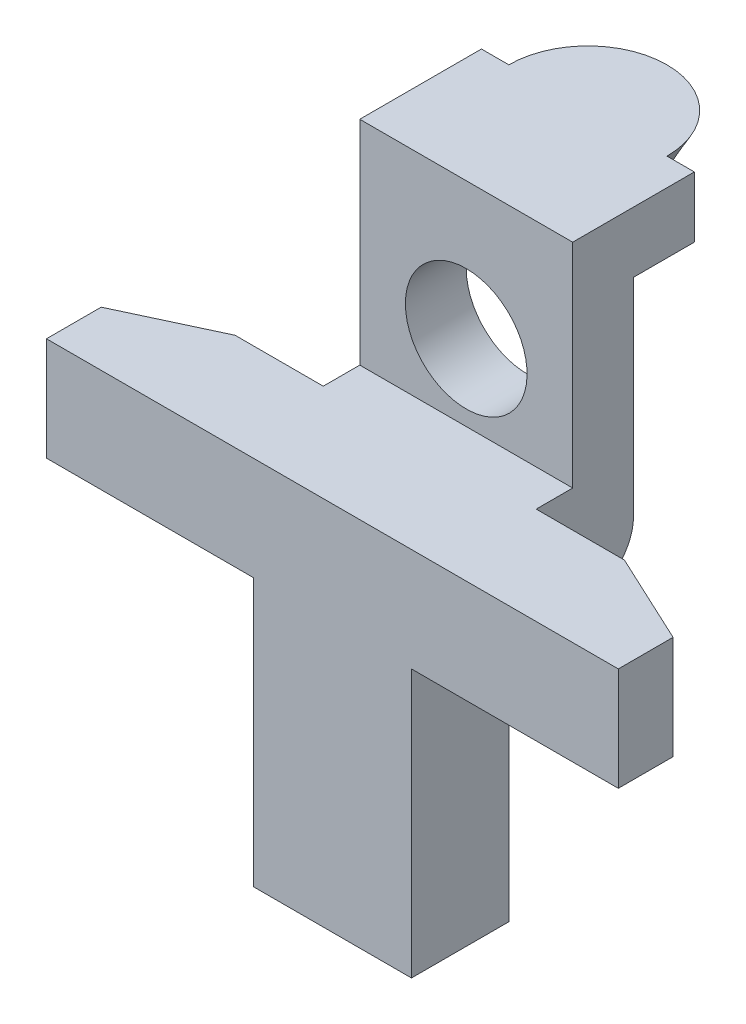
ISO-10303-21;
HEADER;
FILE_DESCRIPTION(('STEP AP214'),'2;1');
FILE_NAME('part.step','',(''),(''),'','','');
FILE_SCHEMA(('AUTOMOTIVE_DESIGN { 1 0 10303 214 1 1 1 1 }'));
ENDSEC;
DATA;
#1=APPLICATION_CONTEXT('core data for automotive mechanical design processes');
#2=APPLICATION_PROTOCOL_DEFINITION('international standard','automotive_design',2000,#1);
#3=PRODUCT_CONTEXT('',#1,'mechanical');
#4=PRODUCT('Part','Part','',(#3));
#5=PRODUCT_RELATED_PRODUCT_CATEGORY('part','',(#4));
#6=PRODUCT_DEFINITION_FORMATION('','',#4);
#7=PRODUCT_DEFINITION_CONTEXT('part definition',#1,'design');
#8=PRODUCT_DEFINITION('design','',#6,#7);
#9=PRODUCT_DEFINITION_SHAPE('','',#8);
#10=(LENGTH_UNIT() NAMED_UNIT(*) SI_UNIT(.MILLI.,.METRE.));
#11=(NAMED_UNIT(*) PLANE_ANGLE_UNIT() SI_UNIT($,.RADIAN.));
#12=(NAMED_UNIT(*) SI_UNIT($,.STERADIAN.) SOLID_ANGLE_UNIT());
#13=UNCERTAINTY_MEASURE_WITH_UNIT(LENGTH_MEASURE(1.E-05),#10,'distance_accuracy_value','');
#14=(GEOMETRIC_REPRESENTATION_CONTEXT(3) GLOBAL_UNCERTAINTY_ASSIGNED_CONTEXT((#13)) GLOBAL_UNIT_ASSIGNED_CONTEXT((#10,
#11,#12)) REPRESENTATION_CONTEXT('',''));
#15=CARTESIAN_POINT('',(0.,0.,0.));
#16=DIRECTION('',(0.,0.,1.));
#17=DIRECTION('',(1.,0.,0.));
#18=AXIS2_PLACEMENT_3D('',#15,#16,#17);
#19=CARTESIAN_POINT('',(17.5,85.9999999999999,-26.));
#20=DIRECTION('',(0.,0.,1.));
#21=DIRECTION('',(1.,0.,0.));
#22=AXIS2_PLACEMENT_3D('',#19,#20,#21);
#23=PLANE('',#22);
#24=DIRECTION('',(-1.,0.,0.));
#25=VECTOR('',#24,1.);
#26=CARTESIAN_POINT('',(17.5,85.9999999999999,-26.));
#27=LINE('',#26,#25);
#28=CARTESIAN_POINT('',(17.5,85.9999999999999,-26.));
#29=VERTEX_POINT('',#28);
#30=CARTESIAN_POINT('',(7.99999999999983,86.,-26.));
#31=VERTEX_POINT('',#30);
#32=EDGE_CURVE('E229',#29,#31,#27,.T.);
#33=ORIENTED_EDGE('',*,*,#32,.T.);
#34=CARTESIAN_POINT('',(7.99999999999982,86.,-26.));
#35=CARTESIAN_POINT('',(8.06461296077254,86.1670097838714,-26.));
#36=CARTESIAN_POINT('',(8.13049843464995,86.33352208519,-26.));
#37=CARTESIAN_POINT('',(8.26459311898194,86.6656013425372,-26.));
#38=CARTESIAN_POINT('',(8.33280223817098,86.8311683353971,-26.));
#39=CARTESIAN_POINT('',(8.54056241212497,87.3264773994168,-26.));
#40=CARTESIAN_POINT('',(8.68327305855971,87.6548962519283,-26.));
#41=CARTESIAN_POINT('',(8.97554544722682,88.3083659231179,-26.));
#42=CARTESIAN_POINT('',(9.12510208396716,88.6334190369549,-26.));
#43=CARTESIAN_POINT('',(9.43000861024656,89.2808110815048,-26.));
#44=CARTESIAN_POINT('',(9.58535880883595,89.6031498662977,-26.));
#45=CARTESIAN_POINT('',(9.99629027719756,90.4396645572338,-26.));
#46=CARTESIAN_POINT('',(10.25567313837,90.9519717419804,-26.));
#47=CARTESIAN_POINT('',(10.7839327016637,91.9717964011415,-26.));
#48=CARTESIAN_POINT('',(11.0528116657692,92.479312697375,-26.));
#49=CARTESIAN_POINT('',(11.5981894834923,93.4909545969185,-26.));
#50=CARTESIAN_POINT('',(11.8746964664123,93.9950758096334,-26.));
#51=CARTESIAN_POINT('',(12.2937311186804,94.7487440257033,-26.));
#52=CARTESIAN_POINT('',(12.4340939451479,94.9994992363485,-26.));
#53=CARTESIAN_POINT('',(12.7161132120268,95.5002785259758,-26.));
#54=CARTESIAN_POINT('',(12.8577696415147,95.7503026111081,-26.));
#55=CARTESIAN_POINT('',(13.0000000000001,95.9999999999999,-26.));
#56=B_SPLINE_CURVE_WITH_KNOTS('',3,(#34,#35,#36,#37,#38,#39,#40,#41,#42,#43,#44,#45,#46,#47,#48,
#49,#50,#51,#52,#53,#54,#55),.UNSPECIFIED.,.F.,.F.,(4,2,2,2,2,2,2,2,2,2,4),(0.,
0.537205746205849,1.07439041691796,2.14853864129819,3.22189845586974,4.29531560961287,
6.01785822993895,7.74081396687128,9.4656828006724,10.3277814664233,11.1898728592339),.UNSPECIFIED.);
#57=CARTESIAN_POINT('',(13.0000000000002,96.,-26.));
#58=VERTEX_POINT('',#57);
#59=EDGE_CURVE('E213',#31,#58,#56,.T.);
#60=ORIENTED_EDGE('',*,*,#59,.T.);
#61=DIRECTION('',(-1.,0.,0.));
#62=VECTOR('',#61,1.);
#63=CARTESIAN_POINT('',(17.5,95.9999999999999,-26.));
#64=LINE('',#63,#62);
#65=CARTESIAN_POINT('',(17.5,95.9999999999999,-26.));
#66=VERTEX_POINT('',#65);
#67=EDGE_CURVE('E227',#66,#58,#64,.T.);
#68=ORIENTED_EDGE('',*,*,#67,.F.);
#69=DIRECTION('',(0.,1.,0.));
#70=VECTOR('',#69,1.);
#71=CARTESIAN_POINT('',(17.5,85.9999999999999,-26.));
#72=LINE('',#71,#70);
#73=EDGE_CURVE('E483',#29,#66,#72,.T.);
#74=ORIENTED_EDGE('',*,*,#73,.F.);
#75=EDGE_LOOP('',(#33,#60,#68,#74));
#76=FACE_BOUND('',#75,.T.);
#77=ADVANCED_FACE('F41',(#76),#23,.F.);
#78=CARTESIAN_POINT('',(0.,0.,0.));
#79=DIRECTION('',(0.,0.,1.));
#80=DIRECTION('',(1.,0.,0.));
#81=AXIS2_PLACEMENT_3D('',#78,#79,#80);
#82=PLANE('',#81);
#83=DIRECTION('',(-1.,0.,0.));
#84=VECTOR('',#83,1.);
#85=CARTESIAN_POINT('',(17.5,44.,0.));
#86=LINE('',#85,#84);
#87=CARTESIAN_POINT('',(13.,44.,0.));
#88=VERTEX_POINT('',#87);
#89=CARTESIAN_POINT('',(-13.,44.,0.));
#90=VERTEX_POINT('',#89);
#91=EDGE_CURVE('E12',#88,#90,#86,.T.);
#92=ORIENTED_EDGE('',*,*,#91,.F.);
#93=DIRECTION('',(0.,1.,0.));
#94=VECTOR('',#93,1.);
#95=CARTESIAN_POINT('',(13.,0.,0.));
#96=LINE('',#95,#94);
#97=CARTESIAN_POINT('',(13.,0.,0.));
#98=VERTEX_POINT('',#97);
#99=EDGE_CURVE('E354',#98,#88,#96,.T.);
#100=ORIENTED_EDGE('',*,*,#99,.F.);
#101=DIRECTION('',(1.,0.,0.));
#102=VECTOR('',#101,1.);
#103=CARTESIAN_POINT('',(0.,0.,0.));
#104=LINE('',#103,#102);
#105=CARTESIAN_POINT('',(8.99999999999999,0.,0.));
#106=VERTEX_POINT('',#105);
#107=EDGE_CURVE('E334',#106,#98,#104,.T.);
#108=ORIENTED_EDGE('',*,*,#107,.F.);
#109=DIRECTION('',(0.,-1.,0.));
#110=VECTOR('',#109,1.);
#111=CARTESIAN_POINT('',(8.99999999999999,0.,0.));
#112=LINE('',#111,#110);
#113=CARTESIAN_POINT('',(9.,25.,0.));
#114=VERTEX_POINT('',#113);
#115=EDGE_CURVE('E327',#114,#106,#112,.T.);
#116=ORIENTED_EDGE('',*,*,#115,.F.);
#117=CARTESIAN_POINT('',(0.,25.,0.));
#118=DIRECTION('',(0.,0.,-1.));
#119=DIRECTION('',(-1.,0.,0.));
#120=AXIS2_PLACEMENT_3D('',#117,#118,#119);
#121=CIRCLE('',#120,9.);
#122=CARTESIAN_POINT('',(-9.,25.,0.));
#123=VERTEX_POINT('',#122);
#124=EDGE_CURVE('E307',#123,#114,#121,.T.);
#125=ORIENTED_EDGE('',*,*,#124,.F.);
#126=DIRECTION('',(0.,1.,0.));
#127=VECTOR('',#126,1.);
#128=CARTESIAN_POINT('',(-9.,25.,0.));
#129=LINE('',#128,#127);
#130=CARTESIAN_POINT('',(-9.,0.,0.));
#131=VERTEX_POINT('',#130);
#132=EDGE_CURVE('E317',#131,#123,#129,.T.);
#133=ORIENTED_EDGE('',*,*,#132,.F.);
#134=CARTESIAN_POINT('',(-13.,0.,0.));
#135=VERTEX_POINT('',#134);
#136=EDGE_CURVE('E346',#135,#131,#104,.T.);
#137=ORIENTED_EDGE('',*,*,#136,.F.);
#138=DIRECTION('',(0.,-1.,0.));
#139=VECTOR('',#138,1.);
#140=CARTESIAN_POINT('',(-13.,44.,0.));
#141=LINE('',#140,#139);
#142=EDGE_CURVE('E344',#90,#135,#141,.T.);
#143=ORIENTED_EDGE('',*,*,#142,.F.);
#144=EDGE_LOOP('',(#92,#100,#108,#116,#125,#133,#137,#143));
#145=FACE_BOUND('',#144,.T.);
#146=ADVANCED_FACE('F370',(#145),#82,.F.);
#147=DIRECTION('',(0.,-1.,0.));
#148=VECTOR('',#147,1.);
#149=CARTESIAN_POINT('',(17.5,44.,0.));
#150=LINE('',#149,#148);
#151=CARTESIAN_POINT('',(17.5,61.,0.));
#152=VERTEX_POINT('',#151);
#153=CARTESIAN_POINT('',(17.5,44.,0.));
#154=VERTEX_POINT('',#153);
#155=EDGE_CURVE('E66',#152,#154,#150,.T.);
#156=ORIENTED_EDGE('',*,*,#155,.F.);
#157=DIRECTION('',(1.,0.,0.));
#158=VECTOR('',#157,1.);
#159=CARTESIAN_POINT('',(13.,61.,0.));
#160=LINE('',#159,#158);
#161=CARTESIAN_POINT('',(32.,61.,0.));
#162=VERTEX_POINT('',#161);
#163=EDGE_CURVE('E306',#152,#162,#160,.T.);
#164=ORIENTED_EDGE('',*,*,#163,.T.);
#165=DIRECTION('',(0.,-1.,0.));
#166=VECTOR('',#165,1.);
#167=CARTESIAN_POINT('',(32.,61.,0.));
#168=LINE('',#167,#166);
#169=CARTESIAN_POINT('',(32.,44.,0.));
#170=VERTEX_POINT('',#169);
#171=EDGE_CURVE('E287',#162,#170,#168,.T.);
#172=ORIENTED_EDGE('',*,*,#171,.T.);
#173=DIRECTION('',(-1.,0.,0.));
#174=VECTOR('',#173,1.);
#175=CARTESIAN_POINT('',(13.,44.,0.));
#176=LINE('',#175,#174);
#177=EDGE_CURVE('E283',#170,#154,#176,.T.);
#178=ORIENTED_EDGE('',*,*,#177,.T.);
#179=EDGE_LOOP('',(#156,#164,#172,#178));
#180=FACE_BOUND('',#179,.T.);
#181=ADVANCED_FACE('F378',(#180),#82,.F.);
#182=CARTESIAN_POINT('',(0.,0.,16.));
#183=DIRECTION('',(0.,1.,0.));
#184=DIRECTION('',(0.,0.,1.));
#185=AXIS2_PLACEMENT_3D('',#182,#183,#184);
#186=PLANE('',#185);
#187=ORIENTED_EDGE('',*,*,#136,.T.);
#188=DIRECTION('',(0.,0.,-1.));
#189=VECTOR('',#188,1.);
#190=CARTESIAN_POINT('',(-9.,0.,12.));
#191=LINE('',#190,#189);
#192=CARTESIAN_POINT('',(-9.,0.,12.));
#193=VERTEX_POINT('',#192);
#194=EDGE_CURVE('E332',#193,#131,#191,.T.);
#195=ORIENTED_EDGE('',*,*,#194,.F.);
#196=DIRECTION('',(-1.,0.,0.));
#197=VECTOR('',#196,1.);
#198=CARTESIAN_POINT('',(-9.,0.,12.));
#199=LINE('',#198,#197);
#200=CARTESIAN_POINT('',(8.99999999999999,0.,12.));
#201=VERTEX_POINT('',#200);
#202=EDGE_CURVE('E316',#201,#193,#199,.T.);
#203=ORIENTED_EDGE('',*,*,#202,.F.);
#204=DIRECTION('',(0.,0.,-1.));
#205=VECTOR('',#204,1.);
#206=CARTESIAN_POINT('',(8.99999999999999,0.,12.));
#207=LINE('',#206,#205);
#208=EDGE_CURVE('E331',#201,#106,#207,.T.);
#209=ORIENTED_EDGE('',*,*,#208,.T.);
#210=ORIENTED_EDGE('',*,*,#107,.T.);
#211=DIRECTION('',(0.,0.,-1.));
#212=VECTOR('',#211,1.);
#213=CARTESIAN_POINT('',(13.,0.,16.));
#214=LINE('',#213,#212);
#215=CARTESIAN_POINT('',(13.,0.,16.));
#216=VERTEX_POINT('',#215);
#217=EDGE_CURVE('E55',#216,#98,#214,.T.);
#218=ORIENTED_EDGE('',*,*,#217,.F.);
#219=DIRECTION('',(1.,0.,0.));
#220=VECTOR('',#219,1.);
#221=CARTESIAN_POINT('',(-13.,0.,16.));
#222=LINE('',#221,#220);
#223=CARTESIAN_POINT('',(-13.,0.,16.));
#224=VERTEX_POINT('',#223);
#225=EDGE_CURVE('E338',#224,#216,#222,.T.);
#226=ORIENTED_EDGE('',*,*,#225,.F.);
#227=DIRECTION('',(0.,0.,-1.));
#228=VECTOR('',#227,1.);
#229=CARTESIAN_POINT('',(-13.,0.,16.));
#230=LINE('',#229,#228);
#231=EDGE_CURVE('E349',#224,#135,#230,.T.);
#232=ORIENTED_EDGE('',*,*,#231,.T.);
#233=EDGE_LOOP('',(#187,#195,#203,#209,#210,#218,#226,#232));
#234=FACE_BOUND('',#233,.T.);
#235=ADVANCED_FACE('F43',(#234),#186,.F.);
#236=CARTESIAN_POINT('',(13.,0.,16.));
#237=DIRECTION('',(-1.,0.,0.));
#238=DIRECTION('',(0.,0.,1.));
#239=AXIS2_PLACEMENT_3D('',#236,#237,#238);
#240=PLANE('',#239);
#241=ORIENTED_EDGE('',*,*,#99,.T.);
#242=DIRECTION('',(0.,0.,1.));
#243=VECTOR('',#242,1.);
#244=CARTESIAN_POINT('',(13.,44.,16.));
#245=LINE('',#244,#243);
#246=CARTESIAN_POINT('',(13.,44.,16.));
#247=VERTEX_POINT('',#246);
#248=EDGE_CURVE('E282',#88,#247,#245,.T.);
#249=ORIENTED_EDGE('',*,*,#248,.T.);
#250=DIRECTION('',(0.,1.,0.));
#251=VECTOR('',#250,1.);
#252=CARTESIAN_POINT('',(13.,0.,16.));
#253=LINE('',#252,#251);
#254=EDGE_CURVE('E345',#216,#247,#253,.T.);
#255=ORIENTED_EDGE('',*,*,#254,.F.);
#256=ORIENTED_EDGE('',*,*,#217,.T.);
#257=EDGE_LOOP('',(#241,#249,#255,#256));
#258=FACE_BOUND('',#257,.T.);
#259=ADVANCED_FACE('F364',(#258),#240,.F.);
#260=CARTESIAN_POINT('',(-13.,44.,16.));
#261=DIRECTION('',(1.,0.,0.));
#262=DIRECTION('',(0.,0.,-1.));
#263=AXIS2_PLACEMENT_3D('',#260,#261,#262);
#264=PLANE('',#263);
#265=DIRECTION('',(0.,-1.,0.));
#266=VECTOR('',#265,1.);
#267=CARTESIAN_POINT('',(-13.,44.,16.));
#268=LINE('',#267,#266);
#269=CARTESIAN_POINT('',(-13.,44.,16.));
#270=VERTEX_POINT('',#269);
#271=EDGE_CURVE('E347',#270,#224,#268,.T.);
#272=ORIENTED_EDGE('',*,*,#271,.F.);
#273=DIRECTION('',(0.,0.,-1.));
#274=VECTOR('',#273,1.);
#275=CARTESIAN_POINT('',(-13.,44.,16.));
#276=LINE('',#275,#274);
#277=EDGE_CURVE('E259',#270,#90,#276,.T.);
#278=ORIENTED_EDGE('',*,*,#277,.T.);
#279=ORIENTED_EDGE('',*,*,#142,.T.);
#280=ORIENTED_EDGE('',*,*,#231,.F.);
#281=EDGE_LOOP('',(#272,#278,#279,#280));
#282=FACE_BOUND('',#281,.T.);
#283=ADVANCED_FACE('F381',(#282),#264,.F.);
#284=CARTESIAN_POINT('',(0.,0.,16.));
#285=DIRECTION('',(0.,0.,1.));
#286=DIRECTION('',(1.,0.,0.));
#287=AXIS2_PLACEMENT_3D('',#284,#285,#286);
#288=PLANE('',#287);
#289=ORIENTED_EDGE('',*,*,#225,.T.);
#290=ORIENTED_EDGE('',*,*,#254,.T.);
#291=DIRECTION('',(1.,0.,0.));
#292=VECTOR('',#291,1.);
#293=CARTESIAN_POINT('',(13.,44.,16.));
#294=LINE('',#293,#292);
#295=CARTESIAN_POINT('',(47.,44.,16.));
#296=VERTEX_POINT('',#295);
#297=EDGE_CURVE('E293',#247,#296,#294,.T.);
#298=ORIENTED_EDGE('',*,*,#297,.T.);
#299=DIRECTION('',(0.,-1.,0.));
#300=VECTOR('',#299,1.);
#301=CARTESIAN_POINT('',(47.,61.,16.));
#302=LINE('',#301,#300);
#303=CARTESIAN_POINT('',(47.,61.,16.));
#304=VERTEX_POINT('',#303);
#305=EDGE_CURVE('E303',#304,#296,#302,.T.);
#306=ORIENTED_EDGE('',*,*,#305,.F.);
#307=DIRECTION('',(1.,0.,0.));
#308=VECTOR('',#307,1.);
#309=CARTESIAN_POINT('',(13.,61.,16.));
#310=LINE('',#309,#308);
#311=CARTESIAN_POINT('',(-47.,61.,15.9999999999999));
#312=VERTEX_POINT('',#311);
#313=EDGE_CURVE('E310',#312,#304,#310,.T.);
#314=ORIENTED_EDGE('',*,*,#313,.F.);
#315=DIRECTION('',(0.,-1.,0.));
#316=VECTOR('',#315,1.);
#317=CARTESIAN_POINT('',(-47.,61.,15.9999999999999));
#318=LINE('',#317,#316);
#319=CARTESIAN_POINT('',(-47.,44.,15.9999999999999));
#320=VERTEX_POINT('',#319);
#321=EDGE_CURVE('E271',#312,#320,#318,.T.);
#322=ORIENTED_EDGE('',*,*,#321,.T.);
#323=DIRECTION('',(1.,0.,0.));
#324=VECTOR('',#323,1.);
#325=CARTESIAN_POINT('',(-13.,44.,16.));
#326=LINE('',#325,#324);
#327=EDGE_CURVE('E257',#320,#270,#326,.T.);
#328=ORIENTED_EDGE('',*,*,#327,.T.);
#329=ORIENTED_EDGE('',*,*,#271,.T.);
#330=EDGE_LOOP('',(#289,#290,#298,#306,#314,#322,#328,#329));
#331=FACE_BOUND('',#330,.T.);
#332=ADVANCED_FACE('F374',(#331),#288,.T.);
#333=CARTESIAN_POINT('',(-32.,61.,0.));
#334=VERTEX_POINT('',#333);
#335=CARTESIAN_POINT('',(-17.5,61.,0.));
#336=VERTEX_POINT('',#335);
#337=EDGE_CURVE('E309',#334,#336,#160,.T.);
#338=ORIENTED_EDGE('',*,*,#337,.T.);
#339=DIRECTION('',(0.,-1.,0.));
#340=VECTOR('',#339,1.);
#341=CARTESIAN_POINT('',(-17.5,44.,0.));
#342=LINE('',#341,#340);
#343=CARTESIAN_POINT('',(-17.5,44.,0.));
#344=VERTEX_POINT('',#343);
#345=EDGE_CURVE('E431',#336,#344,#342,.T.);
#346=ORIENTED_EDGE('',*,*,#345,.T.);
#347=DIRECTION('',(-1.,0.,0.));
#348=VECTOR('',#347,1.);
#349=CARTESIAN_POINT('',(-13.,44.,0.));
#350=LINE('',#349,#348);
#351=CARTESIAN_POINT('',(-32.,44.,0.));
#352=VERTEX_POINT('',#351);
#353=EDGE_CURVE('E261',#344,#352,#350,.T.);
#354=ORIENTED_EDGE('',*,*,#353,.T.);
#355=DIRECTION('',(0.,-1.,0.));
#356=VECTOR('',#355,1.);
#357=CARTESIAN_POINT('',(-32.,61.,0.));
#358=LINE('',#357,#356);
#359=EDGE_CURVE('E279',#334,#352,#358,.T.);
#360=ORIENTED_EDGE('',*,*,#359,.F.);
#361=EDGE_LOOP('',(#338,#346,#354,#360));
#362=FACE_BOUND('',#361,.T.);
#363=ADVANCED_FACE('F390',(#362),#82,.F.);
#364=CARTESIAN_POINT('',(0.,25.,12.));
#365=DIRECTION('',(0.,0.,-1.));
#366=DIRECTION('',(-1.,0.,0.));
#367=AXIS2_PLACEMENT_3D('',#364,#365,#366);
#368=CYLINDRICAL_SURFACE('',#367,9.);
#369=ORIENTED_EDGE('',*,*,#124,.T.);
#370=DIRECTION('',(0.,0.,-1.));
#371=VECTOR('',#370,1.);
#372=CARTESIAN_POINT('',(9.,25.,12.));
#373=LINE('',#372,#371);
#374=CARTESIAN_POINT('',(9.,25.,12.));
#375=VERTEX_POINT('',#374);
#376=EDGE_CURVE('E321',#375,#114,#373,.T.);
#377=ORIENTED_EDGE('',*,*,#376,.F.);
#378=CARTESIAN_POINT('',(0.,25.,12.));
#379=DIRECTION('',(0.,0.,-1.));
#380=DIRECTION('',(-1.,0.,0.));
#381=AXIS2_PLACEMENT_3D('',#378,#379,#380);
#382=CIRCLE('',#381,9.);
#383=CARTESIAN_POINT('',(-9.,25.,12.));
#384=VERTEX_POINT('',#383);
#385=EDGE_CURVE('E315',#384,#375,#382,.T.);
#386=ORIENTED_EDGE('',*,*,#385,.F.);
#387=DIRECTION('',(0.,0.,-1.));
#388=VECTOR('',#387,1.);
#389=CARTESIAN_POINT('',(-9.,25.,12.));
#390=LINE('',#389,#388);
#391=EDGE_CURVE('E328',#384,#123,#390,.T.);
#392=ORIENTED_EDGE('',*,*,#391,.T.);
#393=EDGE_LOOP('',(#369,#377,#386,#392));
#394=FACE_BOUND('',#393,.T.);
#395=ADVANCED_FACE('F725',(#394),#368,.F.);
#396=CARTESIAN_POINT('',(-9.,25.,12.));
#397=DIRECTION('',(-1.,0.,0.));
#398=DIRECTION('',(0.,-1.,0.));
#399=AXIS2_PLACEMENT_3D('',#396,#397,#398);
#400=PLANE('',#399);
#401=ORIENTED_EDGE('',*,*,#132,.T.);
#402=ORIENTED_EDGE('',*,*,#391,.F.);
#403=DIRECTION('',(0.,1.,0.));
#404=VECTOR('',#403,1.);
#405=CARTESIAN_POINT('',(-9.,25.,12.));
#406=LINE('',#405,#404);
#407=EDGE_CURVE('E322',#193,#384,#406,.T.);
#408=ORIENTED_EDGE('',*,*,#407,.F.);
#409=ORIENTED_EDGE('',*,*,#194,.T.);
#410=EDGE_LOOP('',(#401,#402,#408,#409));
#411=FACE_BOUND('',#410,.T.);
#412=ADVANCED_FACE('F713',(#411),#400,.F.);
#413=CARTESIAN_POINT('',(8.99999999999999,0.,12.));
#414=DIRECTION('',(1.,0.,0.));
#415=DIRECTION('',(0.,1.,0.));
#416=AXIS2_PLACEMENT_3D('',#413,#414,#415);
#417=PLANE('',#416);
#418=ORIENTED_EDGE('',*,*,#115,.T.);
#419=ORIENTED_EDGE('',*,*,#208,.F.);
#420=DIRECTION('',(0.,-1.,0.));
#421=VECTOR('',#420,1.);
#422=CARTESIAN_POINT('',(8.99999999999999,0.,12.));
#423=LINE('',#422,#421);
#424=EDGE_CURVE('E314',#375,#201,#423,.T.);
#425=ORIENTED_EDGE('',*,*,#424,.F.);
#426=ORIENTED_EDGE('',*,*,#376,.T.);
#427=EDGE_LOOP('',(#418,#419,#425,#426));
#428=FACE_BOUND('',#427,.T.);
#429=ADVANCED_FACE('F707',(#428),#417,.F.);
#430=CARTESIAN_POINT('',(0.,25.,12.));
#431=DIRECTION('',(0.,0.,-1.));
#432=DIRECTION('',(-1.,0.,0.));
#433=AXIS2_PLACEMENT_3D('',#430,#431,#432);
#434=PLANE('',#433);
#435=ORIENTED_EDGE('',*,*,#385,.T.);
#436=ORIENTED_EDGE('',*,*,#424,.T.);
#437=ORIENTED_EDGE('',*,*,#202,.T.);
#438=ORIENTED_EDGE('',*,*,#407,.T.);
#439=EDGE_LOOP('',(#435,#436,#437,#438));
#440=FACE_BOUND('',#439,.T.);
#441=ADVANCED_FACE('F666',(#440),#434,.T.);
#442=CARTESIAN_POINT('',(13.,61.,16.));
#443=DIRECTION('',(0.,1.,0.));
#444=DIRECTION('',(0.,0.,1.));
#445=AXIS2_PLACEMENT_3D('',#442,#443,#444);
#446=PLANE('',#445);
#447=ORIENTED_EDGE('',*,*,#337,.F.);
#448=DIRECTION('',(-0.906183139995266,0.,0.422885465331122));
#449=VECTOR('',#448,1.);
#450=CARTESIAN_POINT('',(-32.,61.,0.));
#451=LINE('',#450,#449);
#452=CARTESIAN_POINT('',(-47.,61.,6.99999999999994));
#453=VERTEX_POINT('',#452);
#454=EDGE_CURVE('E254',#334,#453,#451,.T.);
#455=ORIENTED_EDGE('',*,*,#454,.T.);
#456=DIRECTION('',(0.,0.,1.));
#457=VECTOR('',#456,1.);
#458=CARTESIAN_POINT('',(-47.,61.,15.9999999999999));
#459=LINE('',#458,#457);
#460=EDGE_CURVE('E268',#453,#312,#459,.T.);
#461=ORIENTED_EDGE('',*,*,#460,.T.);
#462=ORIENTED_EDGE('',*,*,#313,.T.);
#463=DIRECTION('',(0.,0.,-1.));
#464=VECTOR('',#463,1.);
#465=CARTESIAN_POINT('',(47.,61.,16.));
#466=LINE('',#465,#464);
#467=CARTESIAN_POINT('',(47.,61.,7.));
#468=VERTEX_POINT('',#467);
#469=EDGE_CURVE('E285',#304,#468,#466,.T.);
#470=ORIENTED_EDGE('',*,*,#469,.T.);
#471=DIRECTION('',(-0.906183139995265,0.,-0.422885465331124));
#472=VECTOR('',#471,1.);
#473=CARTESIAN_POINT('',(32.,61.,0.));
#474=LINE('',#473,#472);
#475=EDGE_CURVE('E281',#468,#162,#474,.T.);
#476=ORIENTED_EDGE('',*,*,#475,.T.);
#477=ORIENTED_EDGE('',*,*,#163,.F.);
#478=DIRECTION('',(0.,0.,1.));
#479=VECTOR('',#478,1.);
#480=CARTESIAN_POINT('',(17.5,61.,0.));
#481=LINE('',#480,#479);
#482=CARTESIAN_POINT('',(17.5,61.,-6.));
#483=VERTEX_POINT('',#482);
#484=EDGE_CURVE('E457',#483,#152,#481,.T.);
#485=ORIENTED_EDGE('',*,*,#484,.F.);
#486=DIRECTION('',(-1.,0.,0.));
#487=VECTOR('',#486,1.);
#488=CARTESIAN_POINT('',(17.5,61.,-6.));
#489=LINE('',#488,#487);
#490=CARTESIAN_POINT('',(-17.5,61.,-6.));
#491=VERTEX_POINT('',#490);
#492=EDGE_CURVE('E421',#483,#491,#489,.T.);
#493=ORIENTED_EDGE('',*,*,#492,.T.);
#494=DIRECTION('',(0.,0.,1.));
#495=VECTOR('',#494,1.);
#496=CARTESIAN_POINT('',(-17.5,61.,0.));
#497=LINE('',#496,#495);
#498=EDGE_CURVE('E429',#491,#336,#497,.T.);
#499=ORIENTED_EDGE('',*,*,#498,.T.);
#500=EDGE_LOOP('',(#447,#455,#461,#462,#470,#476,#477,#485,#493,#499));
#501=FACE_BOUND('',#500,.T.);
#502=ADVANCED_FACE('F451',(#501),#446,.T.);
#503=CARTESIAN_POINT('',(47.,61.,16.));
#504=DIRECTION('',(-1.,0.,0.));
#505=DIRECTION('',(0.,-1.,0.));
#506=AXIS2_PLACEMENT_3D('',#503,#504,#505);
#507=PLANE('',#506);
#508=DIRECTION('',(0.,0.,-1.));
#509=VECTOR('',#508,1.);
#510=CARTESIAN_POINT('',(47.,44.,16.));
#511=LINE('',#510,#509);
#512=CARTESIAN_POINT('',(47.,44.,7.));
#513=VERTEX_POINT('',#512);
#514=EDGE_CURVE('E291',#296,#513,#511,.T.);
#515=ORIENTED_EDGE('',*,*,#514,.T.);
#516=DIRECTION('',(0.,-1.,0.));
#517=VECTOR('',#516,1.);
#518=CARTESIAN_POINT('',(47.,61.,7.));
#519=LINE('',#518,#517);
#520=EDGE_CURVE('E297',#468,#513,#519,.T.);
#521=ORIENTED_EDGE('',*,*,#520,.F.);
#522=ORIENTED_EDGE('',*,*,#469,.F.);
#523=ORIENTED_EDGE('',*,*,#305,.T.);
#524=EDGE_LOOP('',(#515,#521,#522,#523));
#525=FACE_BOUND('',#524,.T.);
#526=ADVANCED_FACE('F669',(#525),#507,.F.);
#527=CARTESIAN_POINT('',(32.,61.,0.));
#528=DIRECTION('',(-0.422885465331124,0.,0.906183139995265));
#529=DIRECTION('',(0.906183139995266,0.,0.422885465331124));
#530=AXIS2_PLACEMENT_3D('',#527,#528,#529);
#531=PLANE('',#530);
#532=DIRECTION('',(-0.906183139995265,0.,-0.422885465331124));
#533=VECTOR('',#532,1.);
#534=CARTESIAN_POINT('',(32.,44.,0.));
#535=LINE('',#534,#533);
#536=EDGE_CURVE('E294',#513,#170,#535,.T.);
#537=ORIENTED_EDGE('',*,*,#536,.T.);
#538=ORIENTED_EDGE('',*,*,#171,.F.);
#539=ORIENTED_EDGE('',*,*,#475,.F.);
#540=ORIENTED_EDGE('',*,*,#520,.T.);
#541=EDGE_LOOP('',(#537,#538,#539,#540));
#542=FACE_BOUND('',#541,.T.);
#543=ADVANCED_FACE('F679',(#542),#531,.F.);
#544=CARTESIAN_POINT('',(0.,44.,0.));
#545=DIRECTION('',(0.,-1.,0.));
#546=DIRECTION('',(1.,0.,0.));
#547=AXIS2_PLACEMENT_3D('',#544,#545,#546);
#548=PLANE('',#547);
#549=ORIENTED_EDGE('',*,*,#248,.F.);
#550=ORIENTED_EDGE('',*,*,#91,.T.);
#551=ORIENTED_EDGE('',*,*,#277,.F.);
#552=ORIENTED_EDGE('',*,*,#327,.F.);
#553=DIRECTION('',(0.,0.,1.));
#554=VECTOR('',#553,1.);
#555=CARTESIAN_POINT('',(-47.,44.,15.9999999999999));
#556=LINE('',#555,#554);
#557=CARTESIAN_POINT('',(-47.,44.,6.99999999999994));
#558=VERTEX_POINT('',#557);
#559=EDGE_CURVE('E272',#558,#320,#556,.T.);
#560=ORIENTED_EDGE('',*,*,#559,.F.);
#561=DIRECTION('',(-0.906183139995266,0.,0.422885465331122));
#562=VECTOR('',#561,1.);
#563=CARTESIAN_POINT('',(-32.,44.,0.));
#564=LINE('',#563,#562);
#565=EDGE_CURVE('E270',#352,#558,#564,.T.);
#566=ORIENTED_EDGE('',*,*,#565,.F.);
#567=ORIENTED_EDGE('',*,*,#353,.F.);
#568=DIRECTION('',(0.,0.,-1.));
#569=VECTOR('',#568,1.);
#570=CARTESIAN_POINT('',(-17.5,44.,0.));
#571=LINE('',#570,#569);
#572=CARTESIAN_POINT('',(-17.5,44.,-7.99999999999994));
#573=VERTEX_POINT('',#572);
#574=EDGE_CURVE('E436',#344,#573,#571,.T.);
#575=ORIENTED_EDGE('',*,*,#574,.T.);
#576=DIRECTION('',(-1.,0.,0.));
#577=VECTOR('',#576,1.);
#578=CARTESIAN_POINT('',(17.5,44.,-7.99999999999994));
#579=LINE('',#578,#577);
#580=CARTESIAN_POINT('',(17.5,44.,-7.99999999999994));
#581=VERTEX_POINT('',#580);
#582=EDGE_CURVE('E448',#581,#573,#579,.T.);
#583=ORIENTED_EDGE('',*,*,#582,.F.);
#584=DIRECTION('',(0.,0.,-1.));
#585=VECTOR('',#584,1.);
#586=CARTESIAN_POINT('',(17.5,44.,0.));
#587=LINE('',#586,#585);
#588=EDGE_CURVE('E456',#154,#581,#587,.T.);
#589=ORIENTED_EDGE('',*,*,#588,.F.);
#590=ORIENTED_EDGE('',*,*,#177,.F.);
#591=ORIENTED_EDGE('',*,*,#536,.F.);
#592=ORIENTED_EDGE('',*,*,#514,.F.);
#593=ORIENTED_EDGE('',*,*,#297,.F.);
#594=EDGE_LOOP('',(#549,#550,#551,#552,#560,#566,#567,#575,#583,#589,#590,#591,#592,#593));
#595=FACE_BOUND('',#594,.T.);
#596=ADVANCED_FACE('F373',(#595),#548,.T.);
#597=CARTESIAN_POINT('',(-32.,61.,0.));
#598=DIRECTION('',(0.422885465331123,0.,0.906183139995266));
#599=DIRECTION('',(0.906183139995266,0.,-0.422885465331122));
#600=AXIS2_PLACEMENT_3D('',#597,#598,#599);
#601=PLANE('',#600);
#602=ORIENTED_EDGE('',*,*,#565,.T.);
#603=DIRECTION('',(0.,-1.,0.));
#604=VECTOR('',#603,1.);
#605=CARTESIAN_POINT('',(-47.,61.,6.99999999999994));
#606=LINE('',#605,#604);
#607=EDGE_CURVE('E273',#453,#558,#606,.T.);
#608=ORIENTED_EDGE('',*,*,#607,.F.);
#609=ORIENTED_EDGE('',*,*,#454,.F.);
#610=ORIENTED_EDGE('',*,*,#359,.T.);
#611=EDGE_LOOP('',(#602,#608,#609,#610));
#612=FACE_BOUND('',#611,.T.);
#613=ADVANCED_FACE('F647',(#612),#601,.F.);
#614=CARTESIAN_POINT('',(-47.,61.,15.9999999999999));
#615=DIRECTION('',(1.,0.,0.));
#616=DIRECTION('',(0.,1.,0.));
#617=AXIS2_PLACEMENT_3D('',#614,#615,#616);
#618=PLANE('',#617);
#619=ORIENTED_EDGE('',*,*,#559,.T.);
#620=ORIENTED_EDGE('',*,*,#321,.F.);
#621=ORIENTED_EDGE('',*,*,#460,.F.);
#622=ORIENTED_EDGE('',*,*,#607,.T.);
#623=EDGE_LOOP('',(#619,#620,#621,#622));
#624=FACE_BOUND('',#623,.T.);
#625=ADVANCED_FACE('F403',(#624),#618,.F.);
#626=CARTESIAN_POINT('',(17.5,85.9999999999999,-16.));
#627=DIRECTION('',(0.,1.,0.));
#628=DIRECTION('',(0.,0.,1.));
#629=AXIS2_PLACEMENT_3D('',#626,#627,#628);
#630=PLANE('',#629);
#631=CARTESIAN_POINT('',(-7.99999999999983,85.9999999999999,-26.));
#632=VERTEX_POINT('',#631);
#633=CARTESIAN_POINT('',(-17.5,85.9999999999999,-26.));
#634=VERTEX_POINT('',#633);
#635=EDGE_CURVE('E236',#632,#634,#27,.T.);
#636=ORIENTED_EDGE('',*,*,#635,.F.);
#637=CARTESIAN_POINT('',(0.,86.,-26.));
#638=DIRECTION('',(0.,-1.,0.));
#639=DIRECTION('',(0.,0.,-1.));
#640=AXIS2_PLACEMENT_3D('',#637,#638,#639);
#641=CIRCLE('',#640,7.99999999999983);
#642=EDGE_CURVE('E58',#632,#31,#641,.T.);
#643=ORIENTED_EDGE('',*,*,#642,.T.);
#644=ORIENTED_EDGE('',*,*,#32,.F.);
#645=DIRECTION('',(0.,0.,-1.));
#646=VECTOR('',#645,1.);
#647=CARTESIAN_POINT('',(17.5,85.9999999999999,-16.));
#648=LINE('',#647,#646);
#649=CARTESIAN_POINT('',(17.5,85.9999999999999,-16.));
#650=VERTEX_POINT('',#649);
#651=EDGE_CURVE('E445',#650,#29,#648,.T.);
#652=ORIENTED_EDGE('',*,*,#651,.F.);
#653=DIRECTION('',(-1.,0.,0.));
#654=VECTOR('',#653,1.);
#655=CARTESIAN_POINT('',(17.5,85.9999999999999,-16.));
#656=LINE('',#655,#654);
#657=CARTESIAN_POINT('',(-17.5,85.9999999999999,-16.));
#658=VERTEX_POINT('',#657);
#659=EDGE_CURVE('E442',#650,#658,#656,.T.);
#660=ORIENTED_EDGE('',*,*,#659,.T.);
#661=DIRECTION('',(0.,0.,-1.));
#662=VECTOR('',#661,1.);
#663=CARTESIAN_POINT('',(-17.5,85.9999999999999,-16.));
#664=LINE('',#663,#662);
#665=EDGE_CURVE('E466',#658,#634,#664,.T.);
#666=ORIENTED_EDGE('',*,*,#665,.T.);
#667=EDGE_LOOP('',(#636,#643,#644,#652,#660,#666));
#668=FACE_BOUND('',#667,.T.);
#669=ADVANCED_FACE('F400',(#668),#630,.F.);
#670=CARTESIAN_POINT('',(-13.0000000000002,96.,-26.));
#671=VERTEX_POINT('',#670);
#672=CARTESIAN_POINT('',(-17.5,95.9999999999999,-26.));
#673=VERTEX_POINT('',#672);
#674=EDGE_CURVE('E240',#671,#673,#64,.T.);
#675=ORIENTED_EDGE('',*,*,#674,.F.);
#676=CARTESIAN_POINT('',(-13.0000000000001,95.9999999999999,-26.));
#677=CARTESIAN_POINT('',(-12.7698356258625,95.5958731644821,-26.));
#678=CARTESIAN_POINT('',(-12.5411319568445,95.190905648896,-26.));
#679=CARTESIAN_POINT('',(-12.0873509322991,94.3788974445078,-26.));
#680=CARTESIAN_POINT('',(-11.8622739055725,93.971856572084,-26.));
#681=CARTESIAN_POINT('',(-11.4163166820359,93.155059952935,-26.));
#682=CARTESIAN_POINT('',(-11.195439942567,92.7453023148677,-26.));
#683=CARTESIAN_POINT('',(-10.7590591996595,91.9229495004634,-26.));
#684=CARTESIAN_POINT('',(-10.543554994761,91.5103544312672,-26.));
#685=CARTESIAN_POINT('',(-10.1186068969388,90.6806520249872,-26.));
#686=CARTESIAN_POINT('',(-9.90918078796606,90.2635355602095,-26.));
#687=CARTESIAN_POINT('',(-9.4987127748135,89.4253226702227,-26.));
#688=CARTESIAN_POINT('',(-9.29766848517628,89.0042274198026,-26.));
#689=CARTESIAN_POINT('',(-9.00379460488544,88.3684496531001,-26.));
#690=CARTESIAN_POINT('',(-8.90701359033806,88.155591357859,-26.));
#691=CARTESIAN_POINT('',(-8.7164533540151,87.7285384386202,-26.));
#692=CARTESIAN_POINT('',(-8.62267406689129,87.5143438438353,-26.));
#693=CARTESIAN_POINT('',(-8.43845877382712,87.0843952662406,-26.));
#694=CARTESIAN_POINT('',(-8.34802441121901,86.8686405775973,-26.));
#695=CARTESIAN_POINT('',(-8.17100590976297,86.4355396005303,-26.));
#696=CARTESIAN_POINT('',(-8.08442206776867,86.2181931908928,-26.));
#697=CARTESIAN_POINT('',(-7.99999999999983,86.,-26.));
#698=B_SPLINE_CURVE_WITH_KNOTS('',3,(#676,#677,#678,#679,#680,#681,#682,#683,#684,#685,#686,
#687,#688,#689,#690,#691,#692,#693,#694,#695,#696,#697),.UNSPECIFIED.,.F.,.F.,(4,2,2,2,2,2,2,2,
2,2,4),(0.,1.39523135880097,2.79058850904046,4.1870484128255,5.58345587298146,6.98360463634103,
8.3833521600204,9.0848153053152,9.78626316921255,10.4880511907242,11.1898932227121),.UNSPECIFIED.);
#699=EDGE_CURVE('E217',#671,#632,#698,.T.);
#700=ORIENTED_EDGE('',*,*,#699,.T.);
#701=ORIENTED_EDGE('',*,*,#635,.T.);
#702=DIRECTION('',(0.,1.,0.));
#703=VECTOR('',#702,1.);
#704=CARTESIAN_POINT('',(-17.5,85.9999999999999,-26.));
#705=LINE('',#704,#703);
#706=EDGE_CURVE('E408',#634,#673,#705,.T.);
#707=ORIENTED_EDGE('',*,*,#706,.T.);
#708=EDGE_LOOP('',(#675,#700,#701,#707));
#709=FACE_BOUND('',#708,.T.);
#710=ADVANCED_FACE('F388',(#709),#23,.F.);
#711=CARTESIAN_POINT('',(17.5,95.9999999999999,-26.));
#712=DIRECTION('',(0.,-1.,0.));
#713=DIRECTION('',(0.,0.,-1.));
#714=AXIS2_PLACEMENT_3D('',#711,#712,#713);
#715=PLANE('',#714);
#716=ORIENTED_EDGE('',*,*,#67,.T.);
#717=CARTESIAN_POINT('',(0.,96.,-26.));
#718=DIRECTION('',(0.,-1.,0.));
#719=DIRECTION('',(0.,0.,-1.));
#720=AXIS2_PLACEMENT_3D('',#717,#718,#719);
#721=CIRCLE('',#720,13.0000000000002);
#722=EDGE_CURVE('E212',#671,#58,#721,.T.);
#723=ORIENTED_EDGE('',*,*,#722,.F.);
#724=ORIENTED_EDGE('',*,*,#674,.T.);
#725=DIRECTION('',(0.,0.,1.));
#726=VECTOR('',#725,1.);
#727=CARTESIAN_POINT('',(-17.5,95.9999999999999,-26.));
#728=LINE('',#727,#726);
#729=CARTESIAN_POINT('',(-17.5,95.9999999999999,-6.));
#730=VERTEX_POINT('',#729);
#731=EDGE_CURVE('E415',#673,#730,#728,.T.);
#732=ORIENTED_EDGE('',*,*,#731,.T.);
#733=DIRECTION('',(-1.,0.,0.));
#734=VECTOR('',#733,1.);
#735=CARTESIAN_POINT('',(17.5,95.9999999999999,-6.));
#736=LINE('',#735,#734);
#737=CARTESIAN_POINT('',(17.5,95.9999999999999,-6.));
#738=VERTEX_POINT('',#737);
#739=EDGE_CURVE('E239',#738,#730,#736,.T.);
#740=ORIENTED_EDGE('',*,*,#739,.F.);
#741=DIRECTION('',(0.,0.,1.));
#742=VECTOR('',#741,1.);
#743=CARTESIAN_POINT('',(17.5,95.9999999999999,-26.));
#744=LINE('',#743,#742);
#745=EDGE_CURVE('E232',#66,#738,#744,.T.);
#746=ORIENTED_EDGE('',*,*,#745,.F.);
#747=EDGE_LOOP('',(#716,#723,#724,#732,#740,#746));
#748=FACE_BOUND('',#747,.T.);
#749=ADVANCED_FACE('F231',(#748),#715,.F.);
#750=CARTESIAN_POINT('',(17.5,95.9999999999999,-6.));
#751=DIRECTION('',(0.,0.,-1.));
#752=DIRECTION('',(0.,1.,0.));
#753=AXIS2_PLACEMENT_3D('',#750,#751,#752);
#754=PLANE('',#753);
#755=CARTESIAN_POINT('',(0.,73.4999999999999,-6.));
#756=DIRECTION('',(0.,0.,-1.));
#757=DIRECTION('',(0.,1.,0.));
#758=AXIS2_PLACEMENT_3D('',#755,#756,#757);
#759=CIRCLE('',#758,10.);
#760=CARTESIAN_POINT('',(0.,83.4999999999999,-6.));
#761=VERTEX_POINT('',#760);
#762=EDGE_CURVE('E468',#761,#761,#759,.T.);
#763=ORIENTED_EDGE('',*,*,#762,.T.);
#764=EDGE_LOOP('',(#763));
#765=FACE_BOUND('',#764,.T.);
#766=DIRECTION('',(0.,-1.,0.));
#767=VECTOR('',#766,1.);
#768=CARTESIAN_POINT('',(-17.5,95.9999999999999,-6.));
#769=LINE('',#768,#767);
#770=EDGE_CURVE('E419',#730,#491,#769,.T.);
#771=ORIENTED_EDGE('',*,*,#770,.T.);
#772=ORIENTED_EDGE('',*,*,#492,.F.);
#773=DIRECTION('',(0.,-1.,0.));
#774=VECTOR('',#773,1.);
#775=CARTESIAN_POINT('',(17.5,95.9999999999999,-6.));
#776=LINE('',#775,#774);
#777=EDGE_CURVE('E422',#738,#483,#776,.T.);
#778=ORIENTED_EDGE('',*,*,#777,.F.);
#779=ORIENTED_EDGE('',*,*,#739,.T.);
#780=EDGE_LOOP('',(#771,#772,#778,#779));
#781=FACE_BOUND('',#780,.T.);
#782=ADVANCED_FACE('F404',(#765,#781),#754,.F.);
#783=CARTESIAN_POINT('',(17.5,52.,-8.));
#784=DIRECTION('',(-1.,0.,0.));
#785=DIRECTION('',(0.,0.,1.));
#786=AXIS2_PLACEMENT_3D('',#783,#784,#785);
#787=CYLINDRICAL_SURFACE('',#786,8.);
#788=CARTESIAN_POINT('',(-17.5,52.,-8.));
#789=DIRECTION('',(1.,0.,0.));
#790=DIRECTION('',(0.,0.,-1.));
#791=AXIS2_PLACEMENT_3D('',#788,#789,#790);
#792=CIRCLE('',#791,8.);
#793=CARTESIAN_POINT('',(-17.5,52.,-16.));
#794=VERTEX_POINT('',#793);
#795=EDGE_CURVE('E438',#573,#794,#792,.T.);
#796=ORIENTED_EDGE('',*,*,#795,.T.);
#797=DIRECTION('',(-1.,0.,0.));
#798=VECTOR('',#797,1.);
#799=CARTESIAN_POINT('',(17.5,52.,-16.));
#800=LINE('',#799,#798);
#801=CARTESIAN_POINT('',(17.5,52.,-16.));
#802=VERTEX_POINT('',#801);
#803=EDGE_CURVE('E447',#802,#794,#800,.T.);
#804=ORIENTED_EDGE('',*,*,#803,.F.);
#805=CARTESIAN_POINT('',(17.5,52.,-8.));
#806=DIRECTION('',(1.,0.,0.));
#807=DIRECTION('',(0.,0.,-1.));
#808=AXIS2_PLACEMENT_3D('',#805,#806,#807);
#809=CIRCLE('',#808,8.);
#810=EDGE_CURVE('E461',#581,#802,#809,.T.);
#811=ORIENTED_EDGE('',*,*,#810,.F.);
#812=ORIENTED_EDGE('',*,*,#582,.T.);
#813=EDGE_LOOP('',(#796,#804,#811,#812));
#814=FACE_BOUND('',#813,.T.);
#815=ADVANCED_FACE('F497',(#814),#787,.T.);
#816=CARTESIAN_POINT('',(17.5,52.,-16.));
#817=DIRECTION('',(0.,0.,1.));
#818=DIRECTION('',(1.,0.,0.));
#819=AXIS2_PLACEMENT_3D('',#816,#817,#818);
#820=PLANE('',#819);
#821=CARTESIAN_POINT('',(0.,73.4999999999999,-16.));
#822=DIRECTION('',(0.,0.,-1.));
#823=DIRECTION('',(-1.,0.,0.));
#824=AXIS2_PLACEMENT_3D('',#821,#822,#823);
#825=CIRCLE('',#824,10.);
#826=CARTESIAN_POINT('',(-10.,73.4999999999999,-16.));
#827=VERTEX_POINT('',#826);
#828=EDGE_CURVE('E233',#827,#827,#825,.T.);
#829=ORIENTED_EDGE('',*,*,#828,.F.);
#830=EDGE_LOOP('',(#829));
#831=FACE_BOUND('',#830,.T.);
#832=DIRECTION('',(0.,1.,0.));
#833=VECTOR('',#832,1.);
#834=CARTESIAN_POINT('',(-17.5,52.,-16.));
#835=LINE('',#834,#833);
#836=EDGE_CURVE('E439',#794,#658,#835,.T.);
#837=ORIENTED_EDGE('',*,*,#836,.T.);
#838=ORIENTED_EDGE('',*,*,#659,.F.);
#839=DIRECTION('',(0.,1.,0.));
#840=VECTOR('',#839,1.);
#841=CARTESIAN_POINT('',(17.5,52.,-16.));
#842=LINE('',#841,#840);
#843=EDGE_CURVE('E450',#802,#650,#842,.T.);
#844=ORIENTED_EDGE('',*,*,#843,.F.);
#845=ORIENTED_EDGE('',*,*,#803,.T.);
#846=EDGE_LOOP('',(#837,#838,#844,#845));
#847=FACE_BOUND('',#846,.T.);
#848=ADVANCED_FACE('F505',(#831,#847),#820,.F.);
#849=CARTESIAN_POINT('',(17.5,52.,-8.));
#850=DIRECTION('',(1.,0.,0.));
#851=DIRECTION('',(0.,0.,-1.));
#852=AXIS2_PLACEMENT_3D('',#849,#850,#851);
#853=PLANE('',#852);
#854=ORIENTED_EDGE('',*,*,#651,.T.);
#855=ORIENTED_EDGE('',*,*,#73,.T.);
#856=ORIENTED_EDGE('',*,*,#745,.T.);
#857=ORIENTED_EDGE('',*,*,#777,.T.);
#858=ORIENTED_EDGE('',*,*,#484,.T.);
#859=ORIENTED_EDGE('',*,*,#155,.T.);
#860=ORIENTED_EDGE('',*,*,#588,.T.);
#861=ORIENTED_EDGE('',*,*,#810,.T.);
#862=ORIENTED_EDGE('',*,*,#843,.T.);
#863=EDGE_LOOP('',(#854,#855,#856,#857,#858,#859,#860,#861,#862));
#864=FACE_BOUND('',#863,.T.);
#865=ADVANCED_FACE('F484',(#864),#853,.T.);
#866=CARTESIAN_POINT('',(-17.5,52.,-8.));
#867=DIRECTION('',(1.,0.,0.));
#868=DIRECTION('',(0.,0.,-1.));
#869=AXIS2_PLACEMENT_3D('',#866,#867,#868);
#870=PLANE('',#869);
#871=ORIENTED_EDGE('',*,*,#665,.F.);
#872=ORIENTED_EDGE('',*,*,#836,.F.);
#873=ORIENTED_EDGE('',*,*,#795,.F.);
#874=ORIENTED_EDGE('',*,*,#574,.F.);
#875=ORIENTED_EDGE('',*,*,#345,.F.);
#876=ORIENTED_EDGE('',*,*,#498,.F.);
#877=ORIENTED_EDGE('',*,*,#770,.F.);
#878=ORIENTED_EDGE('',*,*,#731,.F.);
#879=ORIENTED_EDGE('',*,*,#706,.F.);
#880=EDGE_LOOP('',(#871,#872,#873,#874,#875,#876,#877,#878,#879));
#881=FACE_BOUND('',#880,.T.);
#882=ADVANCED_FACE('F428',(#881),#870,.F.);
#883=CARTESIAN_POINT('',(0.,73.4999999999999,19.));
#884=DIRECTION('',(0.,0.,-1.));
#885=DIRECTION('',(-1.,0.,0.));
#886=AXIS2_PLACEMENT_3D('',#883,#884,#885);
#887=CYLINDRICAL_SURFACE('',#886,10.);
#888=ORIENTED_EDGE('',*,*,#828,.T.);
#889=EDGE_LOOP('',(#888));
#890=FACE_BOUND('',#889,.T.);
#891=ORIENTED_EDGE('',*,*,#762,.F.);
#892=EDGE_LOOP('',(#891));
#893=FACE_BOUND('',#892,.T.);
#894=ADVANCED_FACE('F508',(#890,#893),#887,.F.);
#895=CARTESIAN_POINT('',(1.05993688171324,96.,-38.9567177096203));
#896=CARTESIAN_POINT('',(-2.65781584350423,86.,-33.5455957314194));
#897=CARTESIAN_POINT('',(26.9733723009539,96.0000000000001,-36.8368439461938));
#898=CARTESIAN_POINT('',(12.4333756193346,86.,-38.8612274184279));
#899=CARTESIAN_POINT('',(24.8534985375274,96.0000000000001,-10.9234085269532));
#900=CARTESIAN_POINT('',(17.7490073063431,86.,-23.770035955589));
#901=CARTESIAN_POINT('',(-1.05993688171324,96.,-13.0432822903797));
#902=CARTESIAN_POINT('',(2.65781584350422,86.,-18.4544042685806));
#903=CARTESIAN_POINT('',(-26.9733723009539,96.0000000000001,-15.1631560538062));
#904=CARTESIAN_POINT('',(-12.4333756193346,86.,-13.1387725815721));
#905=CARTESIAN_POINT('',(-24.8534985375274,96.0000000000001,-41.0765914730468));
#906=CARTESIAN_POINT('',(-17.7490073063431,86.,-28.229964044411));
#907=CARTESIAN_POINT('',(1.05993688171324,96.,-38.9567177096203));
#908=CARTESIAN_POINT('',(-2.65781584350423,86.,-33.5455957314194));
#909=(BOUNDED_SURFACE() B_SPLINE_SURFACE(3,1,((#895,#896),(#897,#898),(#899,#900),(#901,#902),
(#903,#904),(#905,#906),(#907,#908)),.UNSPECIFIED.,.T.,.F.,.F.) B_SPLINE_SURFACE_WITH_KNOTS((4,
3,4),(2,2),(0.,0.5,1.),(0.,1.),
.UNSPECIFIED.) GEOMETRIC_REPRESENTATION_ITEM() RATIONAL_B_SPLINE_SURFACE(((1.,1.),
(0.333333333333333,0.333333333333333),(0.333333333333333,0.333333333333333),(1.,1.),
(0.333333333333333,0.333333333333333),(0.333333333333333,0.333333333333333),(1.,1.))) REPRESENTATION_ITEM('') SURFACE());
#910=CARTESIAN_POINT('',(-1.05993688171324,96.,-13.0432822903797));
#911=CARTESIAN_POINT('',(2.65781584350422,86.,-18.4544042685806));
#912=CARTESIAN_POINT('',(-26.9733723009539,96.0000000000001,-15.1631560538062));
#913=CARTESIAN_POINT('',(-12.4333756193346,86.,-13.1387725815721));
#914=CARTESIAN_POINT('',(-24.8534985375274,96.0000000000001,-41.0765914730468));
#915=CARTESIAN_POINT('',(-17.7490073063431,86.,-28.229964044411));
#916=CARTESIAN_POINT('',(1.05993688171324,96.,-38.9567177096203));
#917=CARTESIAN_POINT('',(-2.65781584350423,86.,-33.5455957314194));
#918=CARTESIAN_POINT('',(26.9733723009539,96.0000000000001,-36.8368439461938));
#919=CARTESIAN_POINT('',(12.4333756193346,86.,-38.8612274184279));
#920=CARTESIAN_POINT('',(24.8534985375274,96.0000000000001,-10.9234085269532));
#921=CARTESIAN_POINT('',(17.7490073063431,86.,-23.770035955589));
#922=CARTESIAN_POINT('',(-1.05993688171324,96.,-13.0432822903797));
#923=CARTESIAN_POINT('',(2.65781584350422,86.,-18.4544042685806));
#924=(BOUNDED_SURFACE() B_SPLINE_SURFACE(3,1,((#910,#911),(#912,#913),(#914,#915),(#916,#917),
(#918,#919),(#920,#921),(#922,#923)),.UNSPECIFIED.,.T.,.F.,.F.) B_SPLINE_SURFACE_WITH_KNOTS((4,
3,4),(2,2),(0.5,1.,1.5),(0.,1.),
.UNSPECIFIED.) GEOMETRIC_REPRESENTATION_ITEM() RATIONAL_B_SPLINE_SURFACE(((1.,1.),
(0.333333333333333,0.333333333333333),(0.333333333333333,0.333333333333333),(1.,1.),
(0.333333333333333,0.333333333333333),(0.333333333333333,0.333333333333333),(1.,1.))) REPRESENTATION_ITEM('') SURFACE());
#925=ORIENTED_EDGE('',*,*,#59,.F.);
#926=ORIENTED_EDGE('',*,*,#642,.F.);
#927=ORIENTED_EDGE('',*,*,#699,.F.);
#928=ORIENTED_EDGE('',*,*,#722,.T.);
#929=EDGE_LOOP('',(#925,#926,#927,#928));
#930=FACE_BOUND('',#929,.T.);
#931=ADVANCED_FACE('F211',(#930),#924,.T.);
#932=CLOSED_SHELL('',(#77,#146,#181,#235,#259,#283,#332,#363,#395,#412,#429,#441,#502,#526,#543,
#596,#613,#625,#669,#710,#749,#782,#815,#848,#865,#882,#894,#931));
#933=MANIFOLD_SOLID_BREP('B2',#932);
#934=ADVANCED_BREP_SHAPE_REPRESENTATION('',(#18,#933),#14);
#935=SHAPE_DEFINITION_REPRESENTATION(#9,#934);
ENDSEC;
END-ISO-10303-21;
